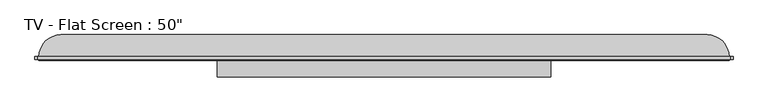
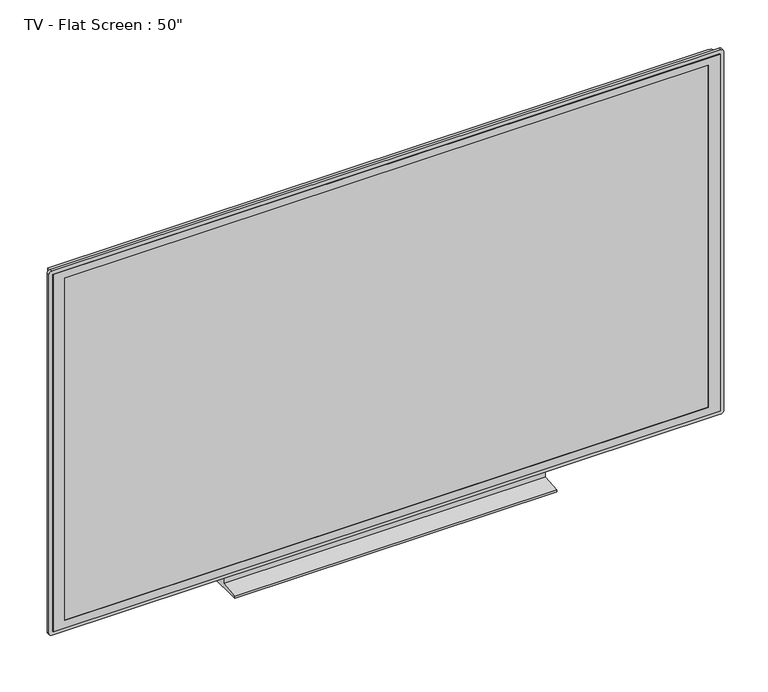
"""IFC4 building model written with IfcOpenShell, lengths in millimetres: furniture geometry."""

from ifc_helpers import new_model, si_unit, point, frame, frame_2d, origin, place, context, project, spatial, polyline, circle_curve, ellipse_curve, trimmed, segment, composite_curve, outline, extrude, faceted_brep, source, transform, mapped, element, save
from ifc_brep_helpers import plane_surface, cylinder_surface, advanced_brep


def furniture_d0237233(model_context):
    return source(origin(), model_context, "Body", "SolidModel", [
        advanced_brep(
        [(-1724.2592928, -51.4613764, 80.0), (1716.3702645, -51.4613764, 80.0), (1716.3702645, -51.4613764, 2028.0255199), (-1724.2592928, -51.4613764, 2028.0255199), (1606.3702645, 58.5386236, 80.0), (-1614.2592928, 58.5386236, 80.0), (-1614.2592928, 58.5386236, 1918.0255199), (1606.3702645, 58.5386236, 1918.0255199)],
        [
            (0, 1),
            (1, 2),
            (2, 3),
            (3, 0),
            (4, 5),
            (5, 6),
            (6, 7),
            (7, 4),
            (0, 5, circle_curve(frame((-1614.2592928, -51.4613764, 80.0), z_axis=(0.0, 0.0, -1.0), x_axis=(-1.0, 0.0, 0.0)), 110.0)),
            (4, 1, circle_curve(frame((1606.3702645, -51.4613764, 80.0), z_axis=(0.0, 0.0, -1.0), x_axis=(1.0, 0.0, 0.0)), 110.0)),
            (7, 2, ellipse_curve(frame((1606.3702645, -51.4613764, 1918.0255199), z_axis=(0.7071067811865475, 0.0, -0.7071067811865475), x_axis=(0.7071067811865474, 0.0, 0.7071067811865476)), 155.5634919, 110.0)),
            (6, 3, ellipse_curve(frame((-1614.2592928, -51.4613764, 1918.0255199), z_axis=(0.7071067811865475, 0.0, 0.7071067811865475), x_axis=(-0.7071067811865476, 0.0, 0.7071067811865474)), 155.5634919, 110.0)),
        ],
        [
            plane_surface(frame((-1724.2592928, -51.4613764, 2028.0255199), z_axis=(0.0, -1.0, 0.0), x_axis=(-1.0, 0.0, 0.0))),
            plane_surface(frame((-1724.2592928, 58.5386236, 2028.0255199), z_axis=(0.0, 1.0, 0.0), x_axis=(1.0, 0.0, 0.0))),
            plane_surface(frame((-1724.2592928, -51.4613764, 80.0), z_axis=(0.0, 0.0, -1.0), x_axis=(0.0, 1.0, 0.0))),
            cylinder_surface(frame((1606.3702645, -51.4613764, 80.0), z_axis=(0.0, 0.0, 1.0), x_axis=(1.0, 0.0, 0.0)), 110.0),
            cylinder_surface(frame((1716.3702645, -51.4613764, 1918.0255199), z_axis=(-1.0, 0.0, 0.0), x_axis=(0.0, 0.0, 1.0)), 110.0),
            cylinder_surface(frame((-1614.2592928, -51.4613764, 2028.0255199), z_axis=(0.0, 0.0, -1.0), x_axis=(-1.0, 0.0, 0.0)), 110.0),
        ],
        [
            (0, [[1, 2, 3, 4]]),
            (1, [[5, 6, 7, 8]]),
            (2, [[-1, 9, -5, 10]]),
            (3, [[11, -2, -10, -8]]),
            (4, [[-11, -7, 12, -3]]),
            (5, [[-12, -6, -9, -4]]),
        ],
    ),
        extrude(outline(composite_curve([segment(polyline([(2048.0255199, 1721.3702645), (2048.0255199, -1729.2592928)]), True, "CONTINUOUS"), segment(trimmed(circle_curve(frame_2d((2033.0255199, -1729.2592928)), 15.0), [point((2048.0255199, -1729.2592928))], [point((2033.0255199, -1744.2592928))], False, "CARTESIAN"), True, "CONTINUOUS"), segment(polyline([(2033.0255199, -1744.2592928), (75.0, -1744.2592928)]), True, "CONTINUOUS"), segment(trimmed(circle_curve(frame_2d((75.0, -1729.2592928)), 15.0), [point((75.0, -1744.2592928))], [point((60.0, -1729.2592928))], False, "CARTESIAN"), True, "CONTINUOUS"), segment(polyline([(60.0, -1729.2592928), (60.0, 1721.3702645)]), True, "CONTINUOUS"), segment(trimmed(circle_curve(frame_2d((75.0, 1721.3702645)), 15.0), [point((60.0, 1721.3702645))], [point((75.0, 1736.3702645))], False, "CARTESIAN"), True, "CONTINUOUS"), segment(polyline([(75.0, 1736.3702645), (2033.0255199, 1736.3702645)]), True, "CONTINUOUS"), segment(trimmed(circle_curve(frame_2d((2033.0255199, 1721.3702645)), 15.0), [point((2033.0255199, 1736.3702645))], [point((2048.0255199, 1721.3702645))], False, "CARTESIAN"), True, "CONTINUOUS")], self_intersect=False), holes=[polyline([(2028.0255199, 1716.3702645), (80.0, 1716.3702645), (80.0, -1724.2592928), (2028.0255199, -1724.2592928), (2028.0255199, 1716.3702645)])]), frame((0.0, -66.4613764, 0.0), z_axis=(0.0, 1.0, 0.0), x_axis=(0.0, 0.0, 1.0)), (0.0, 0.0, 1.0), 15.0),
        faceted_brep([(1716.3702645, -69.4613764, 2028.0255199), (-1724.2592928, -69.4613764, 2028.0255199), (-1724.2592928, -69.4613764, 80.0), (1716.3702645, -69.4613764, 80.0), (-1664.2592928, -69.4613764, 1988.0255199), (1656.3702645, -69.4613764, 1988.0255199), (1656.3702645, -69.4613764, 120.0), (-1664.2592928, -69.4613764, 120.0), (1716.3702645, -51.4613764, 2028.0255199), (1716.3702645, -51.4613764, 80.0), (-1724.2592928, -51.4613764, 80.0), (-1724.2592928, -51.4613764, 2028.0255199), (-1664.2592928, -66.4613764, 1988.0255199), (-1664.2592928, -66.4613764, 120.0), (1656.3702645, -66.4613764, 120.0), (1656.3702645, -66.4613764, 1988.0255199)], [[[0, 1, 2, 3], [4, 5, 6, 7]], [[8, 9, 10, 11]], [[1, 0, 8, 11]], [[2, 1, 11, 10]], [[3, 2, 10, 9]], [[0, 3, 9, 8]], [[12, 13, 14, 15]], [[12, 15, 5, 4]], [[15, 14, 6, 5]], [[14, 13, 7, 6]], [[13, 12, 4, 7]]]),
        extrude(outline(polyline([(-51.4613764, 80.0), (-1.4613764, 80.0), (48.5386236, 0.0), (-151.4613764, 0.0), (-151.4613764, 10.0), (-51.4613764, 20.0), (-51.4613764, 80.0)])), frame((-834.1019035, 0.0, 0.0), z_axis=(1.0, 0.0, 0.0), x_axis=(0.0, 1.0, 0.0)), (0.0, 0.0, 1.0), 1660.3147787),
    ])


if __name__ == "__main__":
    model = new_model("IFC4")
    model_context = context("Model", 3, world=origin())
    ifc_project = project(units=[si_unit("LENGTHUNIT", "METRE", prefix="MILLI")], contexts=[model_context])
    site = spatial("IfcSite", under=ifc_project)
    building = spatial("IfcBuilding", under=site)
    placement = place(None, origin())
    furniture_shape = furniture_d0237233(model_context)
    element("IfcFurniture", 1, ObjectType="TV - Flat Screen : 50\"", at=placement, inside=building, context=model_context, shape_type="MappedRepresentation", body=[
        mapped(furniture_shape, transform((0.0, 0.0, 0.0), x_axis=(1.0, 0.0, 0.0), y_axis=(0.0, 1.0, 0.0), z_axis=(0.0, 0.0, 1.0))),
    ])
    save(model, "model.ifc")

# Revit data of these elements
# Type "TV - Flat Screen : 50\""
#   SinAng = 0' - 0.0193"
#   L = 10' - 10.73345"
#   H = 6' - 1.54431"
#   Thickness = 0' - 4.33071"
#   Diagonal = 12' - 6"
#   CosAng = 0' - 0.03431"
#   Stand [instance default] = yes
#   Default Elevation = 0
# Element 1 (IfcFurniture, "TV - Flat Screen : 50\"")
#   Materials on its faces: "TV - Black", "TV - Glass", "TV - Screen"
# Materials
#   "TV - Black": colour RGB 49 49 49, transparency 0
#   "TV - Glass": colour RGB 157 157 157, transparency 0.9
#   "TV - Screen": colour RGB 0 0 0, transparency 0
